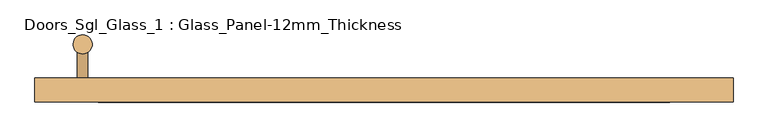
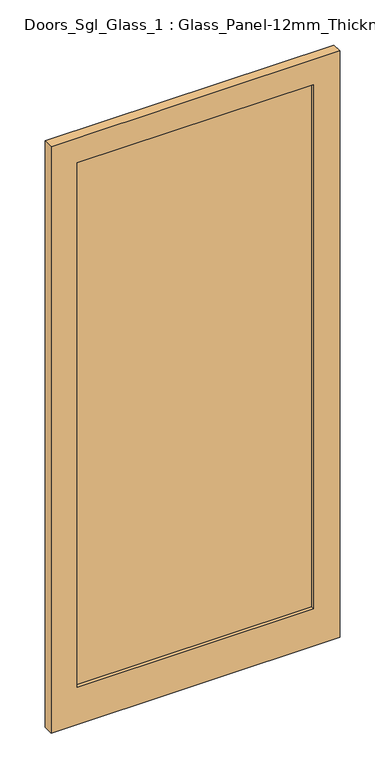
"""IFC4 building model written with IfcOpenShell, lengths in millimetres: door geometry, Doors_Sgl_Glass_1 : Glass_Panel-12mm_Thickness."""

from ifc_helpers import new_model, si_unit, point, frame, frame_2d, origin, place, context, project, spatial, polyline, circle_curve, trimmed, segment, composite_curve, outline, extrude, source, transform, mapped, element, save


def doors_sgl_glass_1_glass_panel_12mm_thickness_ae7dd786(model_context):
    return source(origin(), model_context, "Body", "SweptSolid", [
        extrude(outline(polyline([(449.2712628, 50.0), (449.2712628, 38.0), (-449.2712628, 38.0), (-449.2712628, 50.0), (449.2712628, 50.0)])), frame((0.0, 0.0, 150.0), z_axis=(0.0, 0.0, 1.0), x_axis=(1.0, 0.0, 0.0)), (0.0, 0.0, 1.0), 2105.0),
        extrude(outline(polyline([(0.0, -549.2712628), (0.0, 549.2712628), (2355.0, 549.2712628), (2355.0, -549.2712628), (0.0, -549.2712628)]), holes=[polyline([(2255.0, 449.2712628), (150.0, 449.2712628), (150.0, -449.2712628), (2255.0, -449.2712628), (2255.0, 449.2712628)])]), frame((0.0, 25.0, 0.0), z_axis=(0.0, 1.0, 0.0), x_axis=(0.0, 0.0, 1.0)), (0.0, 0.0, 1.0), 38.0),
        extrude(outline(composite_curve([segment(trimmed(circle_curve(frame_2d((1450.0, -474.2712628)), 8.0), [point((1450.0, -466.2712628))], [point((1450.0, -482.2712628))], False, "CARTESIAN"), True, "CONTINUOUS"), segment(trimmed(circle_curve(frame_2d((1450.0, -474.2712628)), 8.0), [point((1450.0, -482.2712628))], [point((1450.0, -466.2712628))], False, "CARTESIAN"), True, "CONTINUOUS")], self_intersect=False)), frame((0.0, 63.0, 0.0), z_axis=(0.0, 1.0, 0.0), x_axis=(0.0, 0.0, 1.0)), (0.0, 0.0, 1.0), 53.0),
        extrude(outline(composite_curve([segment(trimmed(circle_curve(frame_2d((750.0, -474.2712628)), 8.0), [point((750.0, -466.2712628))], [point((750.0, -482.2712628))], False, "CARTESIAN"), True, "CONTINUOUS"), segment(trimmed(circle_curve(frame_2d((750.0, -474.2712628)), 8.0), [point((750.0, -482.2712628))], [point((750.0, -466.2712628))], False, "CARTESIAN"), True, "CONTINUOUS")], self_intersect=False)), frame((0.0, 63.0, 0.0), z_axis=(0.0, 1.0, 0.0), x_axis=(0.0, 0.0, 1.0)), (0.0, 0.0, 1.0), 53.0),
        extrude(outline(composite_curve([segment(trimmed(circle_curve(frame_2d((-474.2712628, 116.0)), 15.0), [point((-474.2712628, 101.0))], [point((-474.2712628, 131.0))], False, "CARTESIAN"), True, "CONTINUOUS"), segment(trimmed(circle_curve(frame_2d((-474.2712628, 116.0)), 15.0), [point((-474.2712628, 131.0))], [point((-474.2712628, 101.0))], False, "CARTESIAN"), True, "CONTINUOUS")], self_intersect=False)), frame((0.0, 0.0, 650.0), z_axis=(0.0, 0.0, 1.0), x_axis=(1.0, 0.0, 0.0)), (0.0, 0.0, 1.0), 900.0),
    ])


if __name__ == "__main__":
    model = new_model("IFC4")
    model_context = context("Model", 3, world=origin())
    ifc_project = project(units=[si_unit("LENGTHUNIT", "METRE", prefix="MILLI")], contexts=[model_context])
    site = spatial("IfcSite", under=ifc_project)
    building = spatial("IfcBuilding", under=site)
    placement = place(None, origin())
    doors_sgl_glass_1_glass_panel_12mm_thickness_shape = doors_sgl_glass_1_glass_panel_12mm_thickness_ae7dd786(model_context)
    element("IfcDoor", 1, ObjectType="Doors_Sgl_Glass_1 : Glass_Panel-12mm_Thickness", at=placement, inside=building, context=model_context, shape_type="MappedRepresentation", body=[
        mapped(doors_sgl_glass_1_glass_panel_12mm_thickness_shape, transform((0.0, 0.0, 0.0), x_axis=(1.0, 0.0, 0.0), y_axis=(0.0, 1.0, 0.0), z_axis=(0.0, 0.0, 1.0))),
    ])
    save(model, "model.ifc")

# Revit data of these elements
# Type "Doors_Sgl_Glass_1 : Glass_Panel-12mm_Thickness"
#   Type Mark = "60"
#   Construction Type Id = "GSP4R"
#   Keynote = "H11"
#   Analytic Construction = "1/8 in Pilkington single glazing"
#   Visual Light Transmittance = 0.9
#   Stile Top Rail = 0' - 3.93701"
#   Stile Shutting = 0' - 3.93701"
#   Stile Hanging = 0' - 3.93701"
#   Stile Bottom Rail = 0' - 5.90551"
#   Solar Heat Gain Coefficient = 0.78
#   Offset = 0' - 1.9685"
#   Heat Transfer Coefficient (U) = 3.6886 W/(m²·K)
#   Handle X Distance = 0' - 2.95276"
#   Glazing Thickness = 0' - 0.47244"
#   Define Thermal Properties by = 1
#   Material Ironmongery = Metal - Aluminum
#   Material Frame = Metal - Aluminum
#   Material Glass = Glass
#   Function = (empty or 0)
# Element 1 (IfcDoor, "Doors_Sgl_Glass_1 : Glass_Panel-12mm_Thickness")
#   Materials on its faces: "Metal - Aluminum", "Glass"
# Materials
#   "Metal - Aluminum": class "Metal", colour RGB 247 247 247, transparency 0
#   "Glass": class "Glass", colour RGB 0 128 192, transparency 0.9, Description = "Soda Lime Glass", Cost = 0
